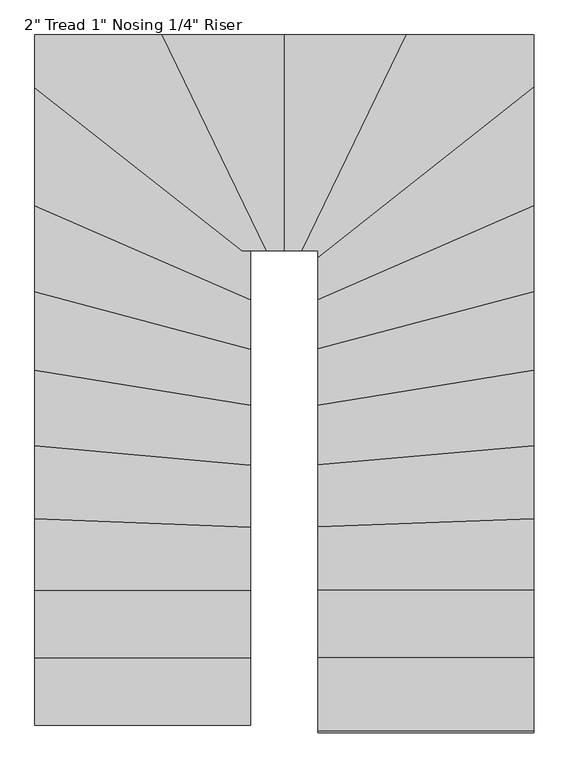
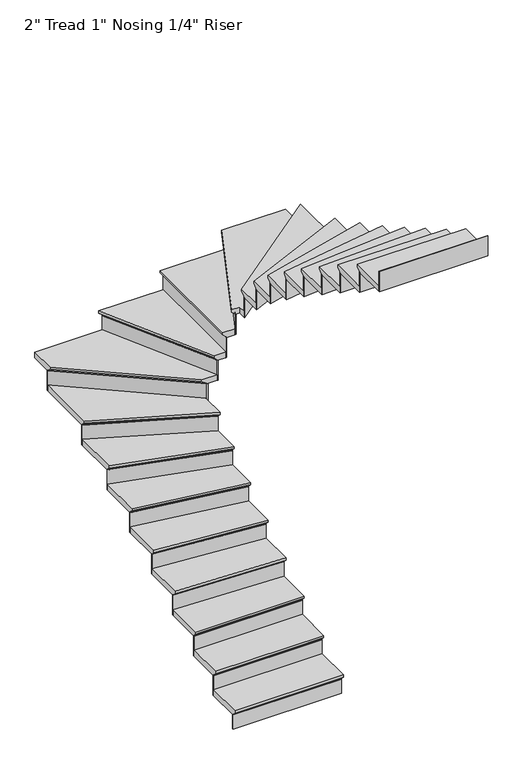
"""IFC4 building model written with IfcOpenShell, lengths in millimetres: stair flight geometry."""

from ifc_helpers import new_model, si_unit, origin, place, context, project, spatial, faceted_brep, source, transform, mapped, element, save


def stair_flight_2efad17c(model_context):
    return source(origin(), model_context, "Body", "Brep", [
        faceted_brep([(-5047.1987704, -4554.2130548, 18443.1214286), (-5047.1987704, -4554.2130548, 18462.1714286), (-5940.8822214, -4554.2130548, 18462.1714286), (-5940.8822214, -4554.2130548, 18443.1214286), (-5047.1987704, -4528.8130548, 18417.7214286), (-5940.8822214, -4528.8130548, 18417.7214286), (-5047.1987704, -4249.4130548, 18462.1714286), (-5940.8822214, -4249.4130548, 18462.1714286), (-5940.8822214, -4528.8130548, 18411.3714286), (-5940.8822214, -4249.4130548, 18411.3714286), (-5047.1987704, -4249.4130548, 18411.3714286), (-5047.1987704, -4528.8130548, 18411.3714286)], [[[0, 1, 2, 3]], [[4, 0, 3, 5]], [[2, 1, 6, 7]], [[8, 9, 10, 11]], [[2, 7, 9, 8, 5, 3]], [[8, 11, 4, 5]], [[6, 1, 0, 4, 11, 10]], [[7, 6, 10, 9]]]),
        faceted_brep([(-5047.1987704, -4528.8130548, 18411.3714286), (-5047.1987704, -4528.8130548, 18288.0), (-5047.1987704, -4522.4630548, 18288.0), (-5047.1987704, -4522.4630548, 18411.3714286), (-5940.8822214, -4528.8130548, 18411.3714286), (-5940.8822214, -4522.4630548, 18411.3714286), (-5940.8822214, -4522.4630548, 18288.0), (-5940.8822214, -4528.8130548, 18288.0)], [[[0, 1, 2, 3]], [[4, 5, 6, 7]], [[1, 0, 4, 7]], [[2, 1, 7, 6]], [[3, 2, 6, 5]], [[0, 3, 5, 4]]]),
        faceted_brep([(-5047.1987704, -4249.4130548, 18585.5428571), (-5047.1987704, -4249.4130548, 18411.3714286), (-5047.1987704, -4243.0630548, 18411.3714286), (-5047.1987704, -4243.0630548, 18585.5428571), (-5940.8822214, -4249.4130548, 18585.5428571), (-5940.8822214, -4243.0630548, 18585.5428571), (-5940.8822214, -4243.0630548, 18411.3714286), (-5940.8822214, -4249.4130548, 18411.3714286)], [[[0, 1, 2, 3]], [[4, 5, 6, 7]], [[1, 0, 4, 7]], [[2, 1, 7, 6]], [[3, 2, 6, 5]], [[0, 3, 5, 4]]]),
        faceted_brep([(-5940.8822214, -4274.8130548, 18636.3428571), (-5047.1987704, -4274.8130548, 18636.3428571), (-5047.1987704, -3970.0130548, 18636.3428571), (-5940.8822214, -3970.0130548, 18636.3428571), (-5940.8822214, -4249.4130548, 18585.5428571), (-5940.8822214, -3970.0130548, 18585.5428571), (-5047.1987704, -3970.0130548, 18585.5428571), (-5047.1987704, -4249.4130548, 18585.5428571), (-5940.8822214, -4249.4130548, 18591.8928571), (-5940.8822214, -4274.8130548, 18617.2928571), (-5047.1987704, -4249.4130548, 18591.8928571), (-5047.1987704, -4274.8130548, 18617.2928571)], [[[0, 1, 2, 3]], [[4, 5, 6, 7]], [[0, 3, 5, 4, 8, 9]], [[4, 7, 10, 8]], [[2, 1, 11, 10, 7, 6]], [[3, 2, 6, 5]], [[11, 1, 0, 9]], [[10, 11, 9, 8]]]),
        faceted_brep([(-5047.1987704, -3970.0130548, 18759.7142857), (-5047.1987704, -3970.0130548, 18585.5428571), (-5047.1987704, -3963.6630548, 18585.5428571), (-5047.1987704, -3963.6630548, 18759.7142857), (-5940.8822214, -3970.0130548, 18759.7142857), (-5940.8822214, -3963.6630548, 18759.7142857), (-5940.8822214, -3963.6630548, 18585.5428571), (-5940.8822214, -3970.0130548, 18585.5428571)], [[[0, 1, 2, 3]], [[4, 5, 6, 7]], [[1, 0, 4, 7]], [[2, 1, 7, 6]], [[3, 2, 6, 5]], [[0, 3, 5, 4]]]),
        faceted_brep([(-5940.8822214, -3995.4130548, 18810.5142857), (-5047.1987704, -3995.4130548, 18810.5142857), (-5047.1987704, -3707.9036879, 18810.5142857), (-5940.8822214, -3673.2843203, 18810.5142857), (-5940.8822214, -3970.0130548, 18759.7142857), (-5940.8822214, -3673.2843203, 18759.7142857), (-5047.1987704, -3707.9036879, 18759.7142857), (-5047.1987704, -3970.0130548, 18759.7142857), (-5940.8822214, -3970.0130548, 18766.0642857), (-5940.8822214, -3995.4130548, 18791.4642857), (-5047.1987704, -3970.0130548, 18766.0642857), (-5047.1987704, -3995.4130548, 18791.4642857)], [[[0, 1, 2, 3]], [[4, 5, 6, 7]], [[0, 3, 5, 4, 8, 9]], [[4, 7, 10, 8]], [[2, 1, 11, 10, 7, 6]], [[3, 2, 6, 5]], [[11, 1, 0, 9]], [[10, 11, 9, 8]]]),
        faceted_brep([(-5047.1987704, -3707.9036879, 18933.8857143), (-5047.1987704, -3707.9036879, 18759.7142857), (-5047.1987704, -3701.5489252, 18759.7142857), (-5047.1987704, -3701.5489252, 18933.8857143), (-5940.8822214, -3673.2843203, 18933.8857143), (-5940.8822214, -3666.9295576, 18933.8857143), (-5940.8822214, -3666.9295576, 18759.7142857), (-5940.8822214, -3673.2843203, 18759.7142857)], [[[0, 1, 2, 3]], [[4, 5, 6, 7]], [[1, 0, 4, 7]], [[2, 1, 7, 6]], [[3, 2, 6, 5]], [[0, 3, 5, 4]]]),
        faceted_brep([(-5940.8822214, -3698.703371, 18984.6857143), (-5047.1987704, -3733.3227386, 18984.6857143), (-5047.1987704, -3451.3234819, 18984.6857143), (-5940.8822214, -3370.89733, 18984.6857143), (-5940.8822214, -3673.2843203, 18933.8857143), (-5940.8822214, -3370.89733, 18933.8857143), (-5047.1987704, -3451.3234819, 18933.8857143), (-5047.1987704, -3707.9036879, 18933.8857143), (-5940.8822214, -3673.2843203, 18940.2357143), (-5940.8822214, -3698.703371, 18965.6357143), (-5047.1987704, -3707.9036879, 18940.2357143), (-5047.1987704, -3733.3227386, 18965.6357143)], [[[0, 1, 2, 3]], [[4, 5, 6, 7]], [[0, 3, 5, 4, 8, 9]], [[4, 7, 10, 8]], [[2, 1, 11, 10, 7, 6]], [[3, 2, 6, 5]], [[11, 1, 0, 9]], [[10, 11, 9, 8]]]),
        faceted_brep([(-5047.1987704, -3451.3234819, 19108.0571429), (-5047.1987704, -3451.3234819, 18933.8857143), (-5047.1987704, -3444.9478197, 18933.8857143), (-5047.1987704, -3444.9478197, 19108.0571429), (-5940.8822214, -3370.89733, 19108.0571429), (-5940.8822214, -3364.5216678, 19108.0571429), (-5940.8822214, -3364.5216678, 18933.8857143), (-5940.8822214, -3370.89733, 18933.8857143)], [[[0, 1, 2, 3]], [[4, 5, 6, 7]], [[1, 0, 4, 7]], [[2, 1, 7, 6]], [[3, 2, 6, 5]], [[0, 3, 5, 4]]]),
        faceted_brep([(-5940.8822214, -3396.3999789, 19158.8571429), (-5047.1987704, -3476.8261308, 19158.8571429), (-5047.1987704, -3203.4301079, 19158.8571429), (-5940.8822214, -3059.5417727, 19158.8571429), (-5940.8822214, -3370.89733, 19108.0571429), (-5940.8822214, -3059.5417727, 19108.0571429), (-5047.1987704, -3203.4301079, 19108.0571429), (-5047.1987704, -3451.3234819, 19108.0571429), (-5940.8822214, -3370.89733, 19114.4071429), (-5940.8822214, -3396.3999789, 19139.8071429), (-5047.1987704, -3451.3234819, 19114.4071429), (-5047.1987704, -3476.8261308, 19139.8071429)], [[[0, 1, 2, 3]], [[4, 5, 6, 7]], [[0, 3, 5, 4, 8, 9]], [[4, 7, 10, 8]], [[2, 1, 11, 10, 7, 6]], [[3, 2, 6, 5]], [[11, 1, 0, 9]], [[10, 11, 9, 8]]]),
        faceted_brep([(-5047.1987704, -3203.4301079, 19282.2285714), (-5047.1987704, -3203.4301079, 19108.0571429), (-5047.1987704, -3196.9983292, 19108.0571429), (-5047.1987704, -3196.9983292, 19282.2285714), (-5940.8822214, -3059.5417727, 19282.2285714), (-5940.8822214, -3053.109994, 19282.2285714), (-5940.8822214, -3053.109994, 19108.0571429), (-5940.8822214, -3059.5417727, 19108.0571429)], [[[0, 1, 2, 3]], [[4, 5, 6, 7]], [[1, 0, 4, 7]], [[2, 1, 7, 6]], [[3, 2, 6, 5]], [[0, 3, 5, 4]]]),
        faceted_brep([(-5940.8822214, -3085.2688872, 19333.0285714), (-5047.1987704, -3229.1572224, 19333.0285714), (-5047.1987704, -2970.3553609, 19333.0285714), (-5940.8822214, -2732.7052783, 19333.0285714), (-5940.8822214, -3059.5417727, 19282.2285714), (-5940.8822214, -2732.7052783, 19282.2285714), (-5047.1987704, -2970.3553609, 19282.2285714), (-5047.1987704, -3203.4301079, 19282.2285714), (-5940.8822214, -3059.5417727, 19288.5785714), (-5940.8822214, -3085.2688872, 19313.9785714), (-5047.1987704, -3203.4301079, 19288.5785714), (-5047.1987704, -3229.1572224, 19313.9785714)], [[[0, 1, 2, 3]], [[4, 5, 6, 7]], [[0, 3, 5, 4, 8, 9]], [[4, 7, 10, 8]], [[2, 1, 11, 10, 7, 6]], [[3, 2, 6, 5]], [[11, 1, 0, 9]], [[10, 11, 9, 8]]]),
        faceted_brep([(-5047.1987704, -2970.3553609, 19456.4), (-5047.1987704, -2970.3553609, 19282.2285714), (-5047.1987704, -2963.7846771, 19282.2285714), (-5047.1987704, -2963.7846771, 19456.4), (-5940.8822214, -2732.7052783, 19456.4), (-5940.8822214, -2726.1345945, 19456.4), (-5940.8822214, -2726.1345945, 19282.2285714), (-5940.8822214, -2732.7052783, 19282.2285714)], [[[0, 1, 2, 3]], [[4, 5, 6, 7]], [[1, 0, 4, 7]], [[2, 1, 7, 6]], [[3, 2, 6, 5]], [[0, 3, 5, 4]]]),
        faceted_brep([(-5940.8822214, -2758.9880136, 19507.2), (-5047.1987704, -2996.6380961, 19507.2), (-5047.1987704, -2765.8050203, 19507.2), (-5940.8822214, -2375.5896532, 19507.2), (-5940.8822214, -2732.7052783, 19456.4), (-5940.8822214, -2375.5896532, 19456.4), (-5047.1987704, -2765.8050203, 19456.4), (-5047.1987704, -2970.3553609, 19456.4), (-5940.8822214, -2732.7052783, 19462.75), (-5940.8822214, -2758.9880136, 19488.15), (-5047.1987704, -2970.3553609, 19462.75), (-5047.1987704, -2996.6380961, 19488.15)], [[[0, 1, 2, 3]], [[4, 5, 6, 7]], [[0, 3, 5, 4, 8, 9]], [[4, 7, 10, 8]], [[2, 1, 11, 10, 7, 6]], [[3, 2, 6, 5]], [[11, 1, 0, 9]], [[10, 11, 9, 8]]]),
        faceted_brep([(-5047.1987704, -2765.8050203, 19630.5714286), (-5047.1987704, -2765.8050203, 19456.4), (-5047.1987704, -2758.8760908, 19456.4), (-5047.1987704, -2758.8760908, 19630.5714286), (-5940.8822214, -2375.5896532, 19630.5714286), (-5940.8822214, -2368.6607237, 19630.5714286), (-5940.8822214, -2368.6607237, 19456.4), (-5940.8822214, -2375.5896532, 19456.4)], [[[0, 1, 2, 3]], [[4, 5, 6, 7]], [[1, 0, 4, 7]], [[2, 1, 7, 6]], [[3, 2, 6, 5]], [[0, 3, 5, 4]]]),
        faceted_brep([(-5940.8822214, -2403.3053713, 19681.3714286), (-5047.1987704, -2793.5207384, 19681.3714286), (-5047.1987704, -2590.8424524, 19681.3714286), (-5040.8038639, -2590.8424524, 19681.3714286), (-5940.8822214, -1882.1944717, 19681.3714286), (-5940.8822214, -2375.5896532, 19630.5714286), (-5940.8822214, -1882.1944717, 19630.5714286), (-5040.8038639, -2590.8424524, 19630.5714286), (-5047.1987704, -2590.8424524, 19630.5714286), (-5047.1987704, -2765.8050203, 19630.5714286), (-5940.8822214, -2375.5896532, 19636.9214286), (-5940.8822214, -2403.3053713, 19662.3214286), (-5047.1987704, -2765.8050203, 19636.9214286), (-5047.1987704, -2793.5207384, 19662.3214286)], [[[0, 1, 2, 3, 4]], [[5, 6, 7, 8, 9]], [[0, 4, 6, 5, 10, 11]], [[5, 9, 12, 10]], [[2, 1, 13, 12, 9, 8]], [[4, 3, 7, 6]], [[13, 1, 0, 11]], [[12, 13, 11, 10]], [[3, 2, 8, 7]]]),
        faceted_brep([(-5040.8038639, -2590.8424524, 19804.7428571), (-5040.8038639, -2590.8424524, 19630.5714286), (-5030.5387554, -2590.8424524, 19630.5714286), (-5030.5387554, -2590.8424524, 19804.7428571), (-5940.8822214, -1882.1944717, 19804.7428571), (-5940.8822214, -1874.1125661, 19804.7428571), (-5940.8822214, -1874.1125661, 19630.5714286), (-5940.8822214, -1882.1944717, 19630.5714286)], [[[0, 1, 2, 3]], [[4, 5, 6, 7]], [[1, 0, 4, 7]], [[2, 1, 7, 6]], [[3, 2, 6, 5]], [[0, 3, 5, 4]]]),
        faceted_brep([(-5384.6489457, -1697.1590014, 19855.5428571), (-5940.8822214, -1697.1590014, 19855.5428571), (-5940.8822214, -1914.5220945, 19855.5428571), (-5081.8642978, -2590.8424524, 19855.5428571), (-4952.3566185, -2590.8424524, 19855.5428571), (-5940.8822214, -1697.1590014, 19804.7428571), (-5384.6489457, -1697.1590014, 19804.7428571), (-4952.3566185, -2590.8424524, 19804.7428571), (-5040.8038639, -2590.8424524, 19804.7428571), (-5940.8822214, -1882.1944717, 19804.7428571), (-5940.8822214, -1882.1944717, 19811.0928571), (-5940.8822214, -1914.5220945, 19836.4928571), (-5040.8038639, -2590.8424524, 19811.0928571), (-5081.8642978, -2590.8424524, 19836.4928571)], [[[0, 1, 2, 3, 4]], [[5, 6, 7, 8, 9]], [[1, 0, 6, 5]], [[2, 1, 5, 9, 10, 11]], [[9, 8, 12, 10]], [[4, 3, 13, 12, 8, 7]], [[0, 4, 7, 6]], [[13, 3, 2, 11]], [[12, 13, 11, 10]]]),
        faceted_brep([(-4952.3566185, -2590.8424524, 19978.9142857), (-4952.3566185, -2590.8424524, 19804.7428571), (-4945.3027294, -2590.8424524, 19804.7428571), (-4945.3027294, -2590.8424524, 19978.9142857), (-5384.6489457, -1697.1590014, 19978.9142857), (-5377.5950566, -1697.1590014, 19978.9142857), (-5377.5950566, -1697.1590014, 19804.7428571), (-5384.6489457, -1697.1590014, 19804.7428571)], [[[0, 1, 2, 3]], [[4, 5, 6, 7]], [[1, 0, 4, 7]], [[2, 1, 7, 6]], [[3, 2, 6, 5]], [[0, 3, 5, 4]]]),
        faceted_brep([(-5412.8645022, -1697.1590014, 20029.7142857), (-4980.5721749, -2590.8424524, 20029.7142857), (-4882.0987704, -2590.8424524, 20029.7142857), (-4882.0987706, -1697.1590014, 20029.7142857), (-5384.6489457, -1697.1590014, 19978.9142857), (-4882.0987706, -1697.1590014, 19978.9142857), (-4882.0987704, -2590.8424524, 19978.9142857), (-4952.3566185, -2590.8424524, 19978.9142857), (-5384.6489457, -1697.1590014, 19985.2642857), (-5412.8645022, -1697.1590014, 20010.6642857), (-4952.3566185, -2590.8424524, 19985.2642857), (-4980.5721749, -2590.8424524, 20010.6642857)], [[[0, 1, 2, 3]], [[4, 5, 6, 7]], [[0, 3, 5, 4, 8, 9]], [[4, 7, 10, 8]], [[3, 2, 6, 5]], [[11, 1, 0, 9]], [[10, 11, 9, 8]], [[2, 1, 11, 10, 7, 6]]]),
        faceted_brep([(-4882.0987704, -2590.8424524, 20153.0857143), (-4882.0987704, -2590.8424524, 19978.9142857), (-4875.7487704, -2590.8424524, 19978.9142857), (-4875.7487704, -2590.8424524, 20153.0857143), (-4882.0987706, -1697.1590014, 20153.0857143), (-4875.7487706, -1697.1590014, 20153.0857143), (-4875.7487706, -1697.1590014, 19978.9142857), (-4882.0987706, -1697.1590014, 19978.9142857)], [[[0, 1, 2, 3]], [[4, 5, 6, 7]], [[1, 0, 4, 7]], [[2, 1, 7, 6]], [[3, 2, 6, 5]], [[0, 3, 5, 4]]]),
        faceted_brep([(-4907.4987706, -1697.1590014, 20203.8857143), (-4907.4987704, -2590.8424524, 20203.8857143), (-4806.2098095, -2590.8424524, 20203.8857143), (-4373.9174828, -1697.1590014, 20203.8857143), (-4882.0987706, -1697.1590014, 20153.0857143), (-4373.9174828, -1697.1590014, 20153.0857143), (-4806.2098095, -2590.8424524, 20153.0857143), (-4882.0987704, -2590.8424524, 20153.0857143), (-4882.0987706, -1697.1590014, 20159.4357143), (-4907.4987706, -1697.1590014, 20184.8357143), (-4882.0987704, -2590.8424524, 20159.4357143), (-4907.4987704, -2590.8424524, 20184.8357143)], [[[0, 1, 2, 3]], [[4, 5, 6, 7]], [[0, 3, 5, 4, 8, 9]], [[4, 7, 10, 8]], [[2, 1, 11, 10, 7, 6]], [[3, 2, 6, 5]], [[11, 1, 0, 9]], [[10, 11, 9, 8]]]),
        faceted_brep([(-4806.2098095, -2590.8424524, 20327.2571429), (-4806.2098095, -2590.8424524, 20153.0857143), (-4799.1559204, -2590.8424524, 20153.0857143), (-4799.1559204, -2590.8424524, 20327.2571429), (-4373.9174828, -1697.1590014, 20327.2571429), (-4366.8635937, -1697.1590014, 20327.2571429), (-4366.8635937, -1697.1590014, 20153.0857143), (-4373.9174828, -1697.1590014, 20153.0857143)], [[[0, 1, 2, 3]], [[4, 5, 6, 7]], [[1, 0, 4, 7]], [[2, 1, 7, 6]], [[3, 2, 6, 5]], [[0, 3, 5, 4]]]),
        faceted_brep([(-3874.1153195, -1946.8497166, 20378.0571429), (-3874.1153195, -1697.1590014, 20378.0571429), (-4402.1330392, -1697.1590014, 20378.0571429), (-4834.4253659, -2590.8424524, 20378.0571429), (-4767.7987704, -2590.8424524, 20378.0571429), (-4767.7987704, -2650.4628721, 20378.0571429), (-3874.1153195, -1697.1590014, 20327.2571429), (-3874.1153195, -1946.8497166, 20327.2571429), (-4767.7987704, -2650.4628721, 20327.2571429), (-4767.7987704, -2590.8424524, 20327.2571429), (-4806.2098095, -2590.8424524, 20327.2571429), (-4373.9174828, -1697.1590014, 20327.2571429), (-4806.2098095, -2590.8424524, 20333.6071429), (-4373.9174828, -1697.1590014, 20333.6071429), (-4834.4253659, -2590.8424524, 20359.0071429), (-4402.1330392, -1697.1590014, 20359.0071429)], [[[0, 1, 2, 3, 4, 5]], [[6, 7, 8, 9, 10, 11]], [[1, 0, 7, 6]], [[11, 10, 12, 13]], [[4, 3, 14, 12, 10, 9]], [[5, 4, 9, 8]], [[0, 5, 8, 7]], [[14, 3, 2, 15]], [[12, 14, 15, 13]], [[2, 1, 6, 11, 13, 15]]]),
        faceted_brep([(-4767.7987704, -2650.4628721, 20501.4285714), (-4767.7987704, -2650.4628721, 20327.2571429), (-4767.7987704, -2658.5447778, 20327.2571429), (-4767.7987704, -2658.5447778, 20501.4285714), (-3874.1153195, -1946.8497166, 20501.4285714), (-3874.1153195, -1954.9316222, 20501.4285714), (-3874.1153195, -1954.9316222, 20327.2571429), (-3874.1153195, -1946.8497166, 20327.2571429)], [[[0, 1, 2, 3]], [[4, 5, 6, 7]], [[1, 0, 4, 7]], [[2, 1, 7, 6]], [[3, 2, 6, 5]], [[0, 3, 5, 4]]]),
        faceted_brep([(-3874.1153195, -1914.5220938, 20552.2285714), (-4767.7987704, -2618.1352494, 20552.2285714), (-4767.7987704, -2821.2364563, 20552.2285714), (-3874.1153195, -2431.0210889, 20552.2285714), (-3874.1153195, -1946.8497166, 20501.4285714), (-3874.1153195, -2431.0210889, 20501.4285714), (-4767.7987704, -2821.2364563, 20501.4285714), (-4767.7987704, -2650.4628721, 20501.4285714), (-3874.1153195, -1946.8497166, 20507.7785714), (-3874.1153195, -1914.5220938, 20533.1785714), (-4767.7987704, -2650.4628721, 20507.7785714), (-4767.7987704, -2618.1352494, 20533.1785714)], [[[0, 1, 2, 3]], [[4, 5, 6, 7]], [[0, 3, 5, 4, 8, 9]], [[4, 7, 10, 8]], [[2, 1, 11, 10, 7, 6]], [[3, 2, 6, 5]], [[11, 1, 0, 9]], [[10, 11, 9, 8]]]),
        faceted_brep([(-4767.7987704, -2821.2364563, 20675.6), (-4767.7987704, -2821.2364563, 20501.4285714), (-4767.7987704, -2828.1653858, 20501.4285714), (-4767.7987704, -2828.1653858, 20675.6), (-3874.1153195, -2431.0210889, 20675.6), (-3874.1153195, -2437.9500185, 20675.6), (-3874.1153195, -2437.9500185, 20501.4285714), (-3874.1153195, -2431.0210889, 20501.4285714)], [[[0, 1, 2, 3]], [[4, 5, 6, 7]], [[1, 0, 4, 7]], [[2, 1, 7, 6]], [[3, 2, 6, 5]], [[0, 3, 5, 4]]]),
        faceted_brep([(-3874.1153195, -2403.3053709, 20726.4), (-4767.7987704, -2793.5207382, 20726.4), (-4767.7987704, -3022.9208311, 20726.4), (-3874.1153195, -2785.2707484, 20726.4), (-3874.1153195, -2431.0210889, 20675.6), (-3874.1153195, -2785.2707484, 20675.6), (-4767.7987704, -3022.9208311, 20675.6), (-4767.7987704, -2821.2364563, 20675.6), (-3874.1153195, -2431.0210889, 20681.95), (-3874.1153195, -2403.3053709, 20707.35), (-4767.7987704, -2821.2364563, 20681.95), (-4767.7987704, -2793.5207382, 20707.35)], [[[0, 1, 2, 3]], [[4, 5, 6, 7]], [[0, 3, 5, 4, 8, 9]], [[4, 7, 10, 8]], [[2, 1, 11, 10, 7, 6]], [[3, 2, 6, 5]], [[11, 1, 0, 9]], [[10, 11, 9, 8]]]),
        faceted_brep([(-4767.7987704, -3022.9208311, 20849.7714286), (-4767.7987704, -3022.9208311, 20675.6), (-4767.7987704, -3029.4915149, 20675.6), (-4767.7987704, -3029.4915149, 20849.7714286), (-3874.1153195, -2785.2707484, 20849.7714286), (-3874.1153195, -2791.8414322, 20849.7714286), (-3874.1153195, -2791.8414322, 20675.6), (-3874.1153195, -2785.2707484, 20675.6)], [[[0, 1, 2, 3]], [[4, 5, 6, 7]], [[1, 0, 4, 7]], [[2, 1, 7, 6]], [[3, 2, 6, 5]], [[0, 3, 5, 4]]]),
        faceted_brep([(-3874.1153195, -2758.9880132, 20900.5714286), (-4767.7987704, -2996.6380959, 20900.5714286), (-4767.7987704, -3254.8843368, 20900.5714286), (-3874.1153195, -3110.9960015, 20900.5714286), (-3874.1153195, -2785.2707484, 20849.7714286), (-3874.1153195, -3110.9960015, 20849.7714286), (-4767.7987704, -3254.8843368, 20849.7714286), (-4767.7987704, -3022.9208311, 20849.7714286), (-3874.1153195, -2785.2707484, 20856.1214286), (-3874.1153195, -2758.9880132, 20881.5214286), (-4767.7987704, -3022.9208311, 20856.1214286), (-4767.7987704, -2996.6380959, 20881.5214286)], [[[0, 1, 2, 3]], [[4, 5, 6, 7]], [[0, 3, 5, 4, 8, 9]], [[4, 7, 10, 8]], [[2, 1, 11, 10, 7, 6]], [[3, 2, 6, 5]], [[11, 1, 0, 9]], [[10, 11, 9, 8]]]),
        faceted_brep([(-4767.7987704, -3254.8843368, 21023.9428571), (-4767.7987704, -3254.8843368, 20849.7714286), (-4767.7987704, -3261.3161154, 20849.7714286), (-4767.7987704, -3261.3161154, 21023.9428571), (-3874.1153195, -3110.9960015, 21023.9428571), (-3874.1153195, -3117.4277801, 21023.9428571), (-3874.1153195, -3117.4277801, 20849.7714286), (-3874.1153195, -3110.9960015, 20849.7714286)], [[[0, 1, 2, 3]], [[4, 5, 6, 7]], [[1, 0, 4, 7]], [[2, 1, 7, 6]], [[3, 2, 6, 5]], [[0, 3, 5, 4]]]),
        faceted_brep([(-3874.1153195, -3085.2688869, 21074.7428571), (-4767.7987704, -3229.1572222, 21074.7428571), (-4767.7987704, -3502.3287795, 21074.7428571), (-3874.1153195, -3421.9026274, 21074.7428571), (-3874.1153195, -3110.9960015, 21023.9428571), (-3874.1153195, -3421.9026274, 21023.9428571), (-4767.7987704, -3502.3287795, 21023.9428571), (-4767.7987704, -3254.8843368, 21023.9428571), (-3874.1153195, -3110.9960015, 21030.2928571), (-3874.1153195, -3085.2688869, 21055.6928571), (-4767.7987704, -3254.8843368, 21030.2928571), (-4767.7987704, -3229.1572222, 21055.6928571)], [[[0, 1, 2, 3]], [[4, 5, 6, 7]], [[0, 3, 5, 4, 8, 9]], [[4, 7, 10, 8]], [[2, 1, 11, 10, 7, 6]], [[3, 2, 6, 5]], [[11, 1, 0, 9]], [[10, 11, 9, 8]]]),
        faceted_brep([(-4767.7987704, -3502.3287795, 21198.1142857), (-4767.7987704, -3502.3287795, 21023.9428571), (-4767.7987704, -3508.7044417, 21023.9428571), (-4767.7987704, -3508.7044417, 21198.1142857), (-3874.1153195, -3421.9026274, 21198.1142857), (-3874.1153195, -3428.2782897, 21198.1142857), (-3874.1153195, -3428.2782897, 21023.9428571), (-3874.1153195, -3421.9026274, 21023.9428571)], [[[0, 1, 2, 3]], [[4, 5, 6, 7]], [[1, 0, 4, 7]], [[2, 1, 7, 6]], [[3, 2, 6, 5]], [[0, 3, 5, 4]]]),
        faceted_brep([(-3874.1153195, -3396.3999786, 21248.9142857), (-4767.7987704, -3476.8261306, 21248.9142857), (-4767.7987704, -3758.7417891, 21248.9142857), (-3874.1153195, -3724.1224215, 21248.9142857), (-3874.1153195, -3421.9026274, 21198.1142857), (-3874.1153195, -3724.1224215, 21198.1142857), (-4767.7987704, -3758.7417891, 21198.1142857), (-4767.7987704, -3502.3287795, 21198.1142857), (-3874.1153195, -3421.9026274, 21204.4642857), (-3874.1153195, -3396.3999786, 21229.8642857), (-4767.7987704, -3502.3287795, 21204.4642857), (-4767.7987704, -3476.8261306, 21229.8642857)], [[[0, 1, 2, 3]], [[4, 5, 6, 7]], [[0, 3, 5, 4, 8, 9]], [[4, 7, 10, 8]], [[2, 1, 11, 10, 7, 6]], [[3, 2, 6, 5]], [[11, 1, 0, 9]], [[10, 11, 9, 8]]]),
        faceted_brep([(-4767.7987704, -3758.7417891, 21372.2857143), (-4767.7987704, -3758.7417891, 21198.1142857), (-4767.7987704, -3765.0965518, 21198.1142857), (-4767.7987704, -3765.0965518, 21372.2857143), (-3874.1153195, -3724.1224215, 21372.2857143), (-3874.1153195, -3730.4771842, 21372.2857143), (-3874.1153195, -3730.4771842, 21198.1142857), (-3874.1153195, -3724.1224215, 21198.1142857)], [[[0, 1, 2, 3]], [[4, 5, 6, 7]], [[1, 0, 4, 7]], [[2, 1, 7, 6]], [[3, 2, 6, 5]], [[0, 3, 5, 4]]]),
        faceted_brep([(-3874.1153195, -3698.7033708, 21423.0857143), (-4767.7987704, -3733.3227384, 21423.0857143), (-4767.7987704, -4020.8130546, 21423.0857143), (-3874.1153195, -4020.8130546, 21423.0857143), (-3874.1153195, -3724.1224215, 21372.2857143), (-3874.1153195, -4020.8130546, 21372.2857143), (-4767.7987704, -4020.8130546, 21372.2857143), (-4767.7987704, -3758.7417891, 21372.2857143), (-3874.1153195, -3724.1224215, 21378.6357143), (-3874.1153195, -3698.7033708, 21404.0357143), (-4767.7987704, -3758.7417891, 21378.6357143), (-4767.7987704, -3733.3227384, 21404.0357143)], [[[0, 1, 2, 3]], [[4, 5, 6, 7]], [[0, 3, 5, 4, 8, 9]], [[4, 7, 10, 8]], [[2, 1, 11, 10, 7, 6]], [[3, 2, 6, 5]], [[11, 1, 0, 9]], [[10, 11, 9, 8]]]),
        faceted_brep([(-4767.7987704, -4020.8130546, 21546.4571429), (-4767.7987704, -4020.8130546, 21372.2857143), (-4767.7987704, -4027.1630546, 21372.2857143), (-4767.7987704, -4027.1630546, 21546.4571429), (-3874.1153195, -4020.8130546, 21546.4571429), (-3874.1153195, -4027.1630546, 21546.4571429), (-3874.1153195, -4027.1630546, 21372.2857143), (-3874.1153195, -4020.8130546, 21372.2857143)], [[[0, 1, 2, 3]], [[4, 5, 6, 7]], [[1, 0, 4, 7]], [[2, 1, 7, 6]], [[3, 2, 6, 5]], [[0, 3, 5, 4]]]),
        faceted_brep([(-3874.1153195, -3995.4130546, 21597.2571429), (-4767.7987704, -3995.4130546, 21597.2571429), (-4767.7987704, -4300.2130546, 21597.2571429), (-3874.1153195, -4300.2130546, 21597.2571429), (-3874.1153195, -4020.8130546, 21546.4571429), (-3874.1153195, -4300.2130546, 21546.4571429), (-4767.7987704, -4300.2130546, 21546.4571429), (-4767.7987704, -4020.8130546, 21546.4571429), (-3874.1153195, -4020.8130546, 21552.8071429), (-3874.1153195, -3995.4130546, 21578.2071429), (-4767.7987704, -4020.8130546, 21552.8071429), (-4767.7987704, -3995.4130546, 21578.2071429)], [[[0, 1, 2, 3]], [[4, 5, 6, 7]], [[0, 3, 5, 4, 8, 9]], [[4, 7, 10, 8]], [[2, 1, 11, 10, 7, 6]], [[3, 2, 6, 5]], [[11, 1, 0, 9]], [[10, 11, 9, 8]]]),
        faceted_brep([(-4767.7987704, -4300.2130546, 21720.6285714), (-4767.7987704, -4300.2130546, 21546.4571429), (-4767.7987704, -4306.5630546, 21546.4571429), (-4767.7987704, -4306.5630546, 21720.6285714), (-3874.1153195, -4300.2130546, 21720.6285714), (-3874.1153195, -4306.5630546, 21720.6285714), (-3874.1153195, -4306.5630546, 21546.4571429), (-3874.1153195, -4300.2130546, 21546.4571429)], [[[0, 1, 2, 3]], [[4, 5, 6, 7]], [[1, 0, 4, 7]], [[2, 1, 7, 6]], [[3, 2, 6, 5]], [[0, 3, 5, 4]]]),
        faceted_brep([(-4767.7987704, -4579.6130546, 21894.8), (-4767.7987704, -4579.6130546, 21720.6285714), (-4767.7987704, -4585.9630546, 21720.6285714), (-4767.7987704, -4585.9630546, 21894.8), (-3874.1153195, -4579.6130546, 21894.8), (-3874.1153195, -4585.9630546, 21894.8), (-3874.1153195, -4585.9630546, 21720.6285714), (-3874.1153195, -4579.6130546, 21720.6285714)], [[[0, 1, 2, 3]], [[4, 5, 6, 7]], [[1, 0, 4, 7]], [[2, 1, 7, 6]], [[3, 2, 6, 5]], [[0, 3, 5, 4]]]),
        faceted_brep([(-3874.1153195, -4274.8130546, 21771.4285714), (-4767.7987704, -4274.8130546, 21771.4285714), (-4767.7987704, -4579.6130546, 21771.4285714), (-3874.1153195, -4579.6130546, 21771.4285714), (-3874.1153195, -4300.2130546, 21720.6285714), (-3874.1153195, -4579.6130546, 21720.6285714), (-4767.7987704, -4579.6130546, 21720.6285714), (-4767.7987704, -4300.2130546, 21720.6285714), (-3874.1153195, -4300.2130546, 21726.9785714), (-3874.1153195, -4274.8130546, 21752.3785714), (-4767.7987704, -4300.2130546, 21726.9785714), (-4767.7987704, -4274.8130546, 21752.3785714)], [[[0, 1, 2, 3]], [[4, 5, 6, 7]], [[0, 3, 5, 4, 8, 9]], [[4, 7, 10, 8]], [[2, 1, 11, 10, 7, 6]], [[3, 2, 6, 5]], [[11, 1, 0, 9]], [[10, 11, 9, 8]]]),
    ])


if __name__ == "__main__":
    model = new_model("IFC4")
    model_context = context("Model", 3, world=origin())
    ifc_project = project(units=[si_unit("LENGTHUNIT", "METRE", prefix="MILLI")], contexts=[model_context])
    site = spatial("IfcSite", under=ifc_project)
    building = spatial("IfcBuilding", under=site)
    placement = place(None, origin())
    stair_flight_shape = stair_flight_2efad17c(model_context)
    element("IfcStairFlight", 1, ObjectType="2\" Tread 1\" Nosing 1/4\" Riser", at=placement, inside=building, context=model_context, shape_type="MappedRepresentation", body=[
        mapped(stair_flight_shape, transform((0.0, 0.0, 0.0), x_axis=(1.0, 0.0, 0.0), y_axis=(0.0, 1.0, 0.0), z_axis=(0.0, 0.0, 1.0))),
    ])
    save(model, "model.ifc")

# Revit data of these elements
# Element 1 (IfcStairFlight, "2\" Tread 1\" Nosing 1/4\" Riser")
#   Materials on its faces: "Tile, Porcelain, 4in"
# Materials
#   "Tile, Porcelain, 4in": class "Generic", colour RGB 89 87 158, transparency 0, Description = "Porcelain tile, 4\", white", Cost = 0
